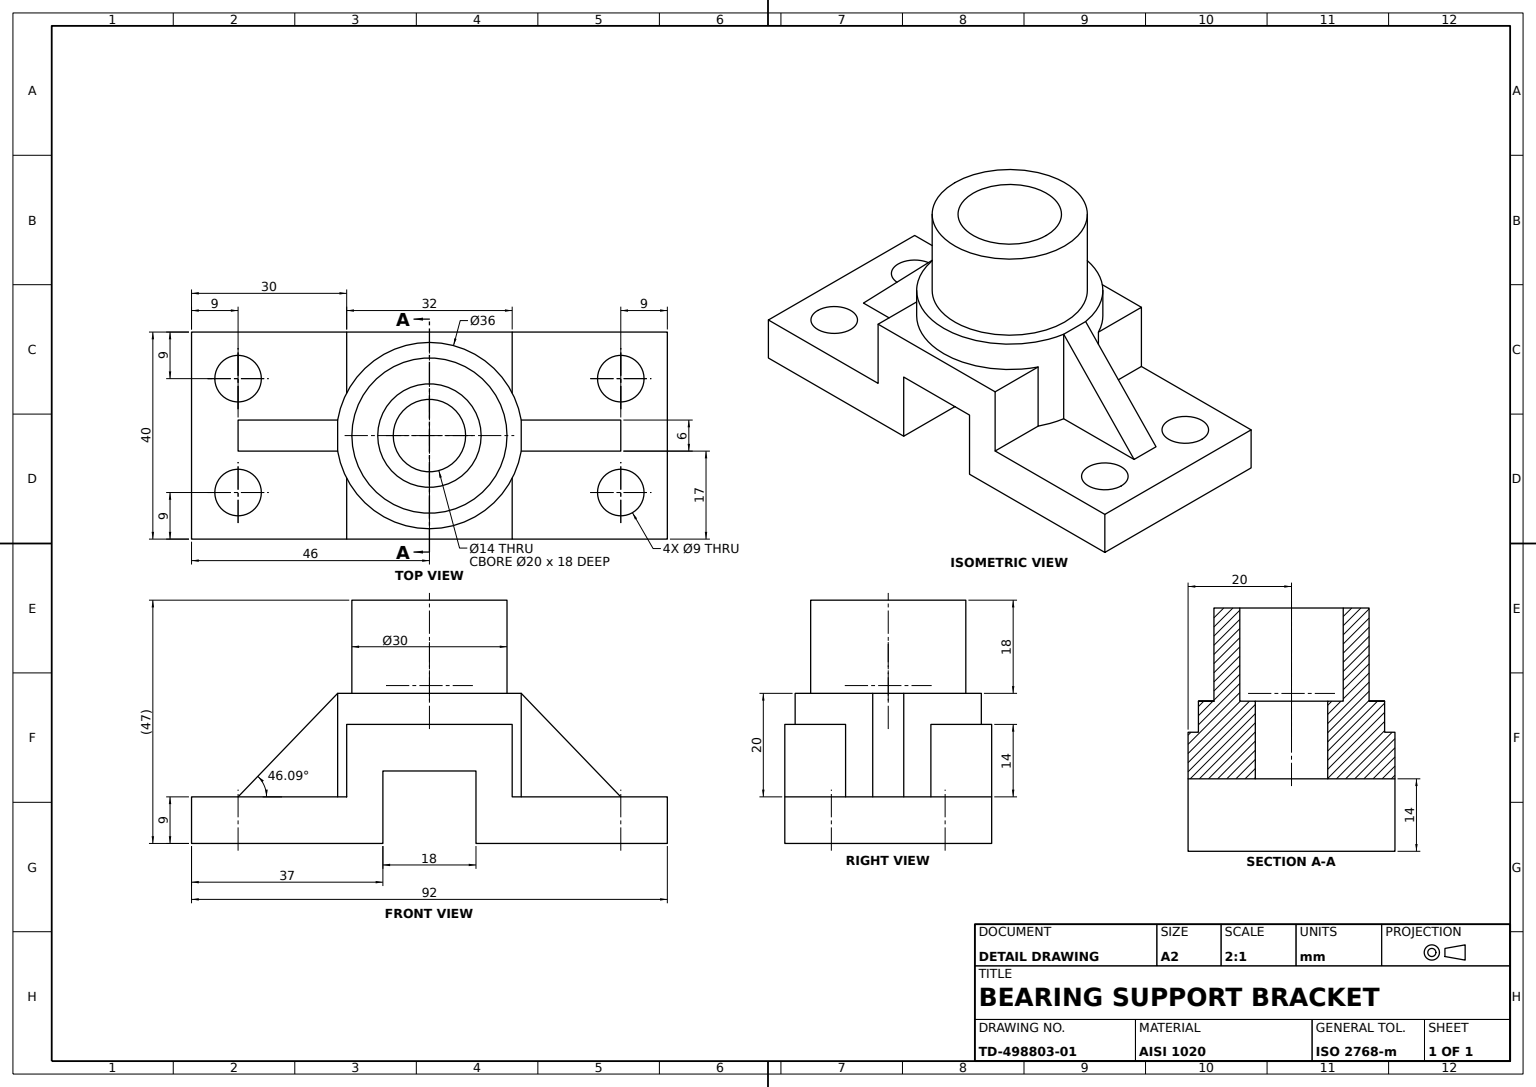
SolidWorks part; units mm, degrees
material "AISI 1020"
ref_plane "Front Plane" through (0, 0, 0) normal (0, 0, 1) x (1, 0, 0)
ref_plane "Top Plane" through (0, 0, 0) normal (0, 1, 0) x (1, 0, 0)
ref_plane "Right Plane" through (0, 0, 0) normal (1, 0, 0) x (0, 0, -1)
sketch "Base Profile Sketch" plane through (0, 0, 0) normal (0, 0, 1) x (1, 0, 0)
  line L0 (0, 0) -> (0, 30.0335) construction
  line L1 (-46, 0) -> (-9, 0)
  line L2 (-9, 0) -> (-9, 14)
  line L3 (-9, 14) -> (9, 14)
  line L4 (9, 14) -> (9, 0)
  line L5 (9, 0) -> (46, 0)
  line L6 (46, 0) -> (46, 9)
  line L7 (46, 9) -> (16, 9)
  line L8 (16, 9) -> (16, 23)
  line L9 (16, 23) -> (-16, 23)
  line L10 (-16, 23) -> (-16, 9)
  line L11 (-16, 9) -> (-46, 9)
  line L12 (-46, 9) -> (-46, 0)
  dimension "D1" = 92
  dimension "D2" = 9
  dimension "D3" = 9
  dimension "D4" = 14
  dimension "D5" = 18
  dimension "D6" = 32
extrude "Stepped Base" add sketch "Base Profile Sketch" along normal mid plane 40
sketch "Collar Ø36 Sketch" plane through (0, 9, 0) normal (0, 1, 0) x (1, 0, 0)
  circle A0 centre (0, 0) radius 18
  dimension "D1" = 36
extrude "Collar Ø36" add sketch "Collar Ø36 Sketch" along normal blind 20
sketch "Collar Trim Sketch" plane through (0, 0, 20) normal (0, 0, 1) x (1, 0, 0)
  line L4 (9, 14) -> (-9, 14)
  line L5 (-9, 14) -> (-9, 9)
  line L6 (-9, 9) -> (9, 9)
  line L7 (9, 9) -> (9, 14)
  line L8 (9, 14) -> (-9, 14)
  line L9 (-9, 14) -> (-9, 9)
  line L10 (-9, 9) -> (9, 9)
  line L11 (9, 9) -> (9, 14)
  dimension "D1" = 0
extrude "Collar Trim Cut" cut sketch "Collar Trim Sketch" against normal through all
sketch "Hub Ø30 Sketch" plane through (0, 29, 0) normal (0, 1, 0) x (1, 0, 0)
  circle A0 centre (0, 0) radius 15
  dimension "D1" = 30
extrude "Hub Ø30" add sketch "Hub Ø30 Sketch" along normal blind 18
sketch "Counterbore Ø20 Sketch" plane through (0, 47, 0) normal (0, 1, 0) x (1, 0, 0)
  circle A0 centre (0, 0) radius 10
  dimension "D1" = 20
extrude "Counterbore Ø20" cut sketch "Counterbore Ø20 Sketch" against normal blind 18
sketch "Bore Ø14 Sketch" plane through (0, 29, 0) normal (0, 1, 0) x (1, 0, 0)
  circle A0 centre (0, 0) radius 7
  dimension "D1" = 14
extrude "Bore Ø14" cut sketch "Bore Ø14 Sketch" against normal through all
sketch "Mounting Hole Ø9 Sketch" plane through (0, 9, 0) normal (0, 1, 0) x (1, 0, 0)
  line L0 (46, -20) -> (46, 20) construction
  line L1 (46, -20) -> (16, -20) construction
  line L2 (0, 0) -> (56.8994, 0) construction
  line L3 (0, 0) -> (0, 29.91) construction
  line L4 (46, 20) -> (16, 20) construction
  circle A0 centre (37, -11) radius 4.5
  circle A1 centre (37, 11) radius 4.5
  dimension "D1" = 9
  dimension "D6" = 9
  dimension "D2" = 9
  dimension "D3" = 9
  dimension "D4" = 9
  dimension "D5" = 9
extrude "Mounting Holes Ø9" cut sketch "Mounting Hole Ø9 Sketch" against normal through all
sketch "Support Rib Sketch" plane through (0, 29, 0) normal (0, 1, 0) x (1, 0, 0)
  line L0 (0, 0) -> (59.6037, 0) construction
  line L1 (37, 3) -> (37, -3)
  line L2 (37, -3) -> (17.7482, -3)
  line L3 (37, 3) -> (17.7482, 3)
  line L4 (46, -20) -> (46, 20) construction
  arc A0 (16, -8.2462) -> (16, 8.2462) centre (0, 0) ccw construction
  arc A1 (17.7482, -3) -> (17.7482, 3) centre (0, 0) ccw
  dimension "D1" = 9
  dimension "D2" = 6
extrude "Support Rib" add sketch "Support Rib Sketch" against normal up to surface (20 mm away) up to face at (32.5, 9, 11)
sketch "Rib Trim Sketch" plane through (0, 0, 3) normal (0, 0, 1) x (1, 0, 0)
  line L0 (17.7482, 29) -> (37, 9)
  line L1 (37, 9) -> (37, 29)
  line L2 (37, 29) -> (17.7482, 29)
extrude "Rib Trim Cut" cut sketch "Rib Trim Sketch" against normal through all
mirror "Rib and Holes Mirror" about plane through (0, 0, 0) normal (1, 0, 0) of "Support Rib", "Mounting Holes Ø9"
sketch "Mirrored Rib Trim Sketch" plane through (0, 0, 3) normal (0, 0, 1) x (1, 0, 0)
  line L0 (-17.7482, 29) -> (-37, 9)
  line L1 (-37, 9) -> (-37, 29)
  line L2 (-37, 29) -> (-17.7482, 29)
extrude "Mirrored Rib Trim Cut" cut sketch "Mirrored Rib Trim Sketch" against normal through all
